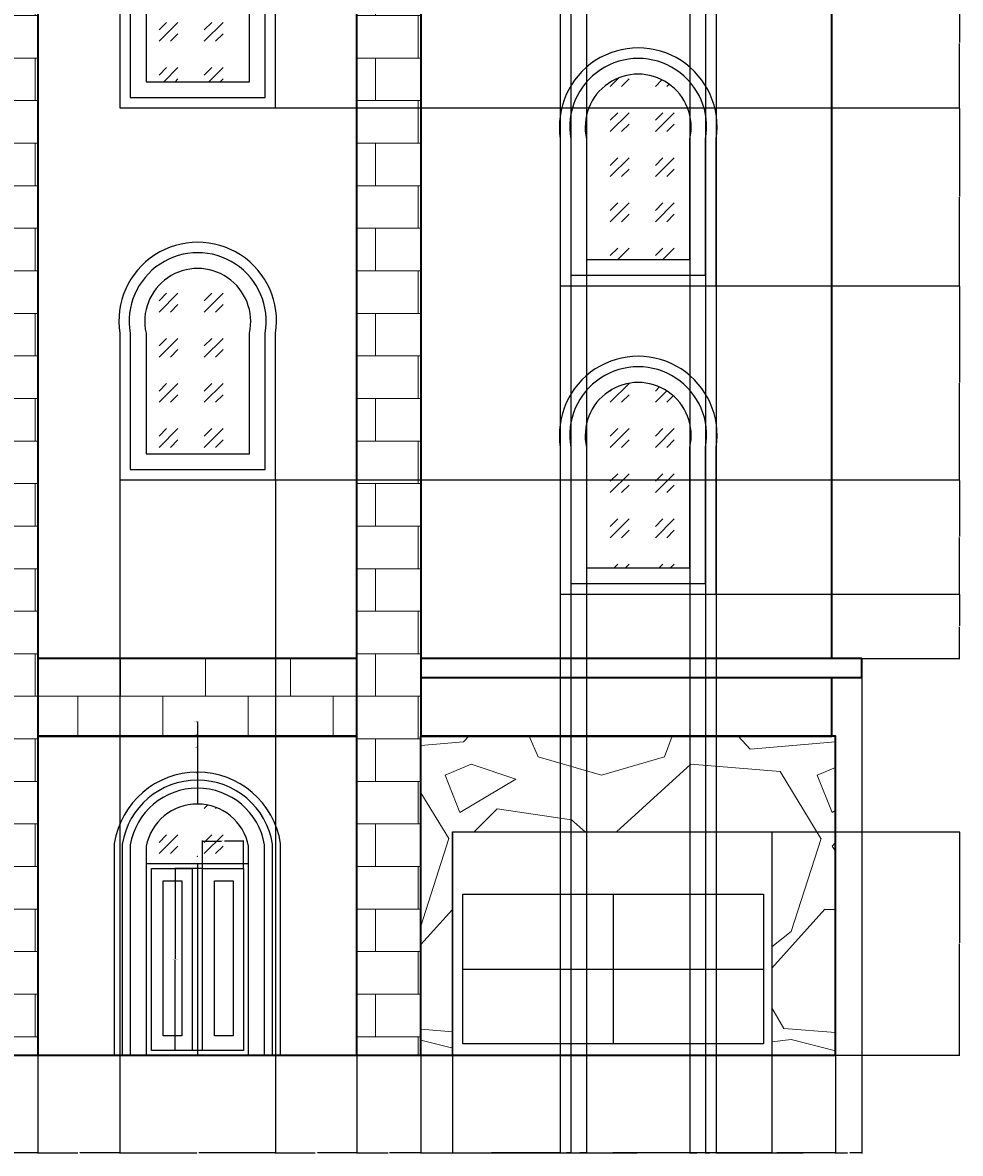
# Model space of a CAD drawing. Units: inches. Extents: x -19 to 556, y -28 to 766.
# Tile 2 of 3: x 203 to 556, y -28 to 397. Entities that reach past the tile are written whole.
import ezdxf

# ---------------------------------------------------------------- set-up
doc = ezdxf.new("R2010")
doc.units = ezdxf.units.IN
doc.header["$MEASUREMENT"] = 0
for name, color, linetype, lineweight in [('A-ANNO-DIMS', 2, 'Continuous', 18), ('A-DOOR', 3, 'Continuous', 25), ('A-ELEV', 7, 'Continuous', 35), ('A-GLAZ', 4, 'Continuous', 25), ('A-GLAZ-PATT', 252, 'Continuous', 13), ('A-WALL-PATT', 8, 'Continuous', 13)]:
    doc.layers.add(name, color=color, linetype=linetype, lineweight=lineweight)
doc.styles.get("Standard").update_dxf_attribs({"font": 'arial.ttf'})
doc.dimstyles.get("Standard").update_dxf_attribs({"dimtxt": 0.18, "dimasz": 0.18, "dimexe": 0.18, "dimexo": 0.0625, "dimgap": 0.09, "dimtad": 0, "dimtih": 1, "dimtoh": 1, "dimdec": 4, "dimzin": 0, "dimdsep": 46, "dimtxsty": 'Standard', "dimcen": 0.09, "dimadec": 0, "dimazin": 0, "dimtfac": 1, "dimtdec": 4, "dimtofl": 0, "dimtmove": 0, "dimatfit": 3, "dimfxl": 1, "dimtolj": 1, "dimtzin": 0, "dimarcsym": 0})
pattern_1 = [(45, (0, 0), (16.97056, 0), [10, -14]), (45, (4.243, 0), (16.97056, 0), [4, -20]), (45, (0, 4.243), (16.97056, 0), [4, -20])]

# ---------------------------------------------------------------- blocks, each defined once
blk = doc.blocks.new('WIN-ARCHED')
for points in [[(65.94, 237.64), (65.94, 182.48), (124.55, 182.48), (124.55, 237.64, 1.168317)], [(69.88, 237.64), (69.88, 186.43), (120.6, 186.43), (120.6, 237.64, 1.194508)], [(75.8, 237.64), (75.8, 192.35), (114.68, 192.35), (114.68, 237.64, 1.253731)]]:
    blk.add_lwpolyline(points, format="xyb", close=True)
blk = doc.blocks.new('DOOR-GARAGE')
for p, q in [((113.34, 69.59), (113.34, 13.35)), ((56.78, 41.47), (169.9, 41.47))]:
    blk.add_line(p, q)
blk.add_lwpolyline([(52.98, 9.07), (52.98, 93.07), (172.98, 93.07), (172.98, 9.07)])
blk.add_lwpolyline([(56.78, 69.59), (169.9, 69.59), (169.9, 13.35), (56.78, 13.35)], close=True)
blk = doc.blocks.new('DOOR-LEAF')
for points in [[(251.66, 79.33), (267.04, 79.33), (267.04, 10.88), (251.66, 10.88)], [(256.13, 74.65), (263.11, 74.65), (263.11, 16.36), (256.13, 16.36)]]:
    blk.add_lwpolyline(points, close=True)
blk = doc.blocks.new('*D6')
at = {"layer": 'A-ANNO-DIMS', "color": 0, "lineweight": -2, "transparency": 16777216}
for p, q in [((270.86, 79.33), (260.47, 79.33)), ((260.65, 79.15), (260.65, 45.29)), ((260.65, 11.06), (260.65, 44.92)), ((270.86, 10.88), (260.47, 10.88))]:
    blk.add_line(p, q, dxfattribs=at)
at = {"layer": 'A-ANNO-DIMS', "color": 0, "transparency": 16777216}
for points in [[(260.62, 79.15), (260.68, 79.15), (260.65, 79.33)], [(260.62, 11.06), (260.68, 11.06), (260.65, 10.88)]]:
    blk.add_solid(points, dxfattribs=at)
at = {"layer": 'Defpoints', "color": 0, "transparency": 16777216}
for p in [(260.65, 79.33), (270.92, 79.33), (270.92, 10.88)]:
    blk.add_point(p, dxfattribs=at)
at = {"layer": 'A-ANNO-DIMS', "color": 0, "transparency": 16777216, "insert": (260.65, 45.1), "char_height": 0.18, "attachment_point": 5}
blk.add_mtext('\\A1;DOOR LEAF 68 TYP.', dxfattribs=at)
blk = doc.blocks.new('*D7')
at = {"layer": 'A-ANNO-DIMS', "color": 0, "lineweight": -2, "transparency": 16777216}
for p, q in [((270.92, 79.39), (270.92, 89.77)), ((271.1, 89.59), (278.09, 89.59)), ((286.12, 89.59), (279.13, 89.59)), ((286.3, 79.39), (286.3, 89.77))]:
    blk.add_line(p, q, dxfattribs=at)
at = {"layer": 'A-ANNO-DIMS', "color": 0, "transparency": 16777216}
for points in [[(271.1, 89.62), (271.1, 89.56), (270.92, 89.59)], [(286.12, 89.62), (286.12, 89.56), (286.3, 89.59)]]:
    blk.add_solid(points, dxfattribs=at)
at = {"layer": 'Defpoints', "color": 0, "transparency": 16777216}
for p in [(286.3, 89.59), (270.92, 79.33), (286.3, 79.33)]:
    blk.add_point(p, dxfattribs=at)
at = {"layer": 'A-ANNO-DIMS', "color": 0, "transparency": 16777216, "insert": (278.61, 89.59), "char_height": 0.18, "attachment_point": 5}
blk.add_mtext('\\A1;15 TYP.', dxfattribs=at)
blk = doc.blocks.new('*D17')
at = {"layer": 'A-ANNO-DIMS', "color": 0, "lineweight": -2, "transparency": 16777216}
for p, q in [((485.05, 93.07), (555.75, 93.07)), ((555.57, 92.89), (555.57, 51.26)), ((555.57, 9.25), (555.57, 50.89)), ((485.05, 9.07), (555.75, 9.07))]:
    blk.add_line(p, q, dxfattribs=at)
at = {"layer": 'A-ANNO-DIMS', "color": 0, "transparency": 16777216}
for points in [[(555.54, 92.89), (555.6, 92.89), (555.57, 93.07)], [(555.54, 9.25), (555.6, 9.25), (555.57, 9.07)]]:
    blk.add_solid(points, dxfattribs=at)
at = {"layer": 'Defpoints', "color": 0, "transparency": 16777216}
for p in [(484.98, 93.07), (555.57, 93.07), (484.98, 9.07)]:
    blk.add_point(p, dxfattribs=at)
at = {"layer": 'A-ANNO-DIMS', "color": 0, "transparency": 16777216, "insert": (555.57, 51.07), "char_height": 0.18, "attachment_point": 5}
blk.add_mtext('\\A1;84', dxfattribs=at)
blk = doc.blocks.new('*D18')
at = {"layer": 'A-ANNO-DIMS', "color": 0, "lineweight": -2, "transparency": 16777216}
for p, q in [((364.98, 93.01), (364.98, -27.86)), ((484.98, 93.01), (484.98, -27.86)), ((365.16, -27.68), (424.7, -27.68)), ((484.8, -27.68), (425.26, -27.68))]:
    blk.add_line(p, q, dxfattribs=at)
at = {"layer": 'A-ANNO-DIMS', "color": 0, "transparency": 16777216}
for points in [[(365.16, -27.65), (365.16, -27.71), (364.98, -27.68)], [(484.8, -27.65), (484.8, -27.71), (484.98, -27.68)]]:
    blk.add_solid(points, dxfattribs=at)
at = {"layer": 'Defpoints', "color": 0, "transparency": 16777216}
for p in [(364.98, 93.07), (484.98, 93.07), (484.98, -27.68)]:
    blk.add_point(p, dxfattribs=at)
at = {"layer": 'A-ANNO-DIMS', "color": 0, "transparency": 16777216, "insert": (424.98, -27.68), "char_height": 0.18, "attachment_point": 5}
blk.add_mtext('\\A1;120', dxfattribs=at)
blk = doc.blocks.new('*D21')
at = {"layer": 'A-ANNO-DIMS', "color": 0, "lineweight": -2, "transparency": 16777216}
for p, q in [((484.98, 9.01), (484.98, -27.86)), ((508.98, 9.01), (508.98, -27.86)), ((485.16, -27.68), (496.76, -27.68)), ((508.8, -27.68), (497.2, -27.68))]:
    blk.add_line(p, q, dxfattribs=at)
at = {"layer": 'A-ANNO-DIMS', "color": 0, "transparency": 16777216}
for points in [[(485.16, -27.65), (485.16, -27.71), (484.98, -27.68)], [(508.8, -27.65), (508.8, -27.71), (508.98, -27.68)]]:
    blk.add_solid(points, dxfattribs=at)
at = {"layer": 'Defpoints', "color": 0, "transparency": 16777216}
for p in [(484.98, 9.07), (508.98, 9.07), (508.98, -27.68)]:
    blk.add_point(p, dxfattribs=at)
at = {"layer": 'A-ANNO-DIMS', "color": 0, "transparency": 16777216, "insert": (496.98, -27.68), "char_height": 0.18, "attachment_point": 5}
blk.add_mtext('\\A1;24', dxfattribs=at)
blk = doc.blocks.new('*D22')
at = {"layer": 'A-ANNO-DIMS', "color": 0, "lineweight": -2, "transparency": 16777216}
for p, q in [((464.13, 182.48), (555.75, 182.48)), ((555.57, 182.3), (555.57, 170.55)), ((555.57, 158.44), (555.57, 170.19)), ((507.68, 158.26), (555.75, 158.26))]:
    blk.add_line(p, q, dxfattribs=at)
at = {"layer": 'A-ANNO-DIMS', "color": 0, "transparency": 16777216}
for points in [[(555.54, 182.3), (555.6, 182.3), (555.57, 182.48)], [(555.54, 158.44), (555.6, 158.44), (555.57, 158.26)]]:
    blk.add_solid(points, dxfattribs=at)
at = {"layer": 'Defpoints', "color": 0, "transparency": 16777216}
for p in [(464.07, 182.48), (555.57, 182.48), (507.61, 158.26)]:
    blk.add_point(p, dxfattribs=at)
at = {"layer": 'A-ANNO-DIMS', "color": 0, "transparency": 16777216, "insert": (555.57, 170.37), "char_height": 0.18, "attachment_point": 5}
blk.add_mtext('\\A1;24.223', dxfattribs=at)
blk = doc.blocks.new('*D23')
at = {"layer": 'A-ANNO-DIMS', "color": 0, "lineweight": -2, "transparency": 16777216}
for p, q in [((298.45, 225.36), (555.75, 225.36)), ((555.57, 225.18), (555.57, 204.1)), ((555.57, 182.66), (555.57, 203.74)), ((464.13, 182.48), (555.75, 182.48))]:
    blk.add_line(p, q, dxfattribs=at)
at = {"layer": 'A-ANNO-DIMS', "color": 0, "transparency": 16777216}
for points in [[(555.54, 225.18), (555.6, 225.18), (555.57, 225.36)], [(555.54, 182.66), (555.6, 182.66), (555.57, 182.48)]]:
    blk.add_solid(points, dxfattribs=at)
at = {"layer": 'Defpoints', "color": 0, "transparency": 16777216}
for p in [(298.39, 225.36), (555.57, 225.36), (464.07, 182.48)]:
    blk.add_point(p, dxfattribs=at)
at = {"layer": 'A-ANNO-DIMS', "color": 0, "transparency": 16777216, "insert": (555.57, 203.92), "char_height": 0.18, "attachment_point": 5}
blk.add_mtext('\\A1;42.88', dxfattribs=at)
blk = doc.blocks.new('*D24')
at = {"layer": 'A-ANNO-DIMS', "color": 0, "lineweight": -2, "transparency": 16777216}
for p, q in [((464.13, 298.43), (555.75, 298.43)), ((555.57, 298.25), (555.57, 262.08)), ((555.57, 225.54), (555.57, 261.71)), ((298.45, 225.36), (555.75, 225.36))]:
    blk.add_line(p, q, dxfattribs=at)
at = {"layer": 'A-ANNO-DIMS', "color": 0, "transparency": 16777216}
for points in [[(555.54, 298.25), (555.6, 298.25), (555.57, 298.43)], [(555.54, 225.54), (555.6, 225.54), (555.57, 225.36)]]:
    blk.add_solid(points, dxfattribs=at)
at = {"layer": 'Defpoints', "color": 0, "transparency": 16777216}
for p in [(464.07, 298.43), (555.57, 298.43), (298.39, 225.36)]:
    blk.add_point(p, dxfattribs=at)
at = {"layer": 'A-ANNO-DIMS', "color": 0, "transparency": 16777216, "insert": (555.57, 261.89), "char_height": 0.18, "attachment_point": 5}
blk.add_mtext('\\A1;73.06', dxfattribs=at)
blk = doc.blocks.new('*D25')
at = {"layer": 'A-ANNO-DIMS', "color": 0, "lineweight": -2, "transparency": 16777216}
for p, q in [((298.45, 365.25), (555.75, 365.25)), ((555.57, 365.07), (555.57, 332.02)), ((555.57, 298.61), (555.57, 331.66)), ((464.13, 298.43), (555.75, 298.43))]:
    blk.add_line(p, q, dxfattribs=at)
at = {"layer": 'A-ANNO-DIMS', "color": 0, "transparency": 16777216}
for points in [[(555.54, 365.07), (555.6, 365.07), (555.57, 365.25)], [(555.54, 298.61), (555.6, 298.61), (555.57, 298.43)]]:
    blk.add_solid(points, dxfattribs=at)
at = {"layer": 'Defpoints', "color": 0, "transparency": 16777216}
for p in [(298.39, 365.25), (555.57, 365.25), (464.07, 298.43)]:
    blk.add_point(p, dxfattribs=at)
at = {"layer": 'A-ANNO-DIMS', "color": 0, "transparency": 16777216, "insert": (555.57, 331.84), "char_height": 0.18, "attachment_point": 5}
blk.add_mtext('\\A1;66.83', dxfattribs=at)
blk = doc.blocks.new('*D26')
at = {"layer": 'A-ANNO-DIMS', "color": 0, "lineweight": -2, "transparency": 16777216}
for p, q in [((464.13, 414.2), (555.75, 414.2)), ((555.57, 414.02), (555.57, 389.91)), ((555.57, 365.43), (555.57, 389.55)), ((298.45, 365.25), (555.75, 365.25))]:
    blk.add_line(p, q, dxfattribs=at)
at = {"layer": 'A-ANNO-DIMS', "color": 0, "transparency": 16777216}
for points in [[(555.54, 414.02), (555.6, 414.02), (555.57, 414.2)], [(555.54, 365.43), (555.6, 365.43), (555.57, 365.25)]]:
    blk.add_solid(points, dxfattribs=at)
at = {"layer": 'Defpoints', "color": 0, "transparency": 16777216}
for p in [(464.07, 414.2), (555.57, 414.2), (298.39, 365.25)]:
    blk.add_point(p, dxfattribs=at)
at = {"layer": 'A-ANNO-DIMS', "color": 0, "transparency": 16777216, "insert": (555.57, 389.73), "char_height": 0.18, "attachment_point": 5}
blk.add_mtext('\\A1;48.95', dxfattribs=at)
blk = doc.blocks.new('*D33')
at = {"layer": 'A-ANNO-DIMS', "color": 0, "lineweight": -2, "transparency": 16777216}
for p, q in [((184.98, 9.01), (184.98, -27.86)), ((208.98, 9.01), (208.98, -27.86)), ((185.16, -27.68), (196.76, -27.68)), ((208.8, -27.68), (197.2, -27.68))]:
    blk.add_line(p, q, dxfattribs=at)
at = {"layer": 'A-ANNO-DIMS', "color": 0, "transparency": 16777216}
for points in [[(185.16, -27.65), (185.16, -27.71), (184.98, -27.68)], [(208.8, -27.65), (208.8, -27.71), (208.98, -27.68)]]:
    blk.add_solid(points, dxfattribs=at)
at = {"layer": 'Defpoints', "color": 0, "transparency": 16777216}
for p in [(184.98, 9.07), (208.98, 9.07), (208.98, -27.68)]:
    blk.add_point(p, dxfattribs=at)
at = {"layer": 'A-ANNO-DIMS', "color": 0, "transparency": 16777216, "insert": (196.98, -27.68), "char_height": 0.18, "attachment_point": 5}
blk.add_mtext('\\A1;24', dxfattribs=at)
blk = doc.blocks.new('*D34')
at = {"layer": 'A-ANNO-DIMS', "color": 0, "lineweight": -2, "transparency": 16777216}
for p, q in [((239.78, 225.3), (239.78, -27.86)), ((208.98, 9.01), (208.98, -27.86)), ((209.16, -27.68), (223.99, -27.68)), ((239.6, -27.68), (224.77, -27.68))]:
    blk.add_line(p, q, dxfattribs=at)
at = {"layer": 'A-ANNO-DIMS', "color": 0, "transparency": 16777216}
for points in [[(209.16, -27.65), (209.16, -27.71), (208.98, -27.68)], [(239.6, -27.65), (239.6, -27.71), (239.78, -27.68)]]:
    blk.add_solid(points, dxfattribs=at)
at = {"layer": 'Defpoints', "color": 0, "transparency": 16777216}
for p in [(239.78, 225.36), (208.98, 9.07), (239.78, -27.68)]:
    blk.add_point(p, dxfattribs=at)
at = {"layer": 'A-ANNO-DIMS', "color": 0, "transparency": 16777216, "insert": (224.38, -27.68), "char_height": 0.18, "attachment_point": 5}
blk.add_mtext('\\A1;30.79', dxfattribs=at)
blk = doc.blocks.new('*D35')
at = {"layer": 'A-ANNO-DIMS', "color": 0, "lineweight": -2, "transparency": 16777216}
for p, q in [((239.78, 225.3), (239.78, -27.86)), ((298.39, 225.3), (298.39, -27.86)), ((239.96, -27.68), (268.71, -27.68)), ((298.21, -27.68), (269.46, -27.68))]:
    blk.add_line(p, q, dxfattribs=at)
at = {"layer": 'A-ANNO-DIMS', "color": 0, "transparency": 16777216}
for points in [[(239.96, -27.65), (239.96, -27.71), (239.78, -27.68)], [(298.21, -27.65), (298.21, -27.71), (298.39, -27.68)]]:
    blk.add_solid(points, dxfattribs=at)
at = {"layer": 'Defpoints', "color": 0, "transparency": 16777216}
for p in [(239.78, 225.36), (298.39, 225.36), (298.39, -27.68)]:
    blk.add_point(p, dxfattribs=at)
at = {"layer": 'A-ANNO-DIMS', "color": 0, "transparency": 16777216, "insert": (269.08, -27.68), "char_height": 0.18, "attachment_point": 5}
blk.add_mtext('\\A1;58.61', dxfattribs=at)
blk = doc.blocks.new('*D36')
at = {"layer": 'A-ANNO-DIMS', "color": 0, "lineweight": -2, "transparency": 16777216}
for p, q in [((298.39, 225.3), (298.39, -27.86)), ((328.98, 9.01), (328.98, -27.86)), ((298.57, -27.68), (313.22, -27.68)), ((328.8, -27.68), (314.15, -27.68))]:
    blk.add_line(p, q, dxfattribs=at)
at = {"layer": 'A-ANNO-DIMS', "color": 0, "transparency": 16777216}
for points in [[(298.57, -27.65), (298.57, -27.71), (298.39, -27.68)], [(328.8, -27.65), (328.8, -27.71), (328.98, -27.68)]]:
    blk.add_solid(points, dxfattribs=at)
at = {"layer": 'Defpoints', "color": 0, "transparency": 16777216}
for p in [(298.39, 225.36), (328.98, 9.07), (328.98, -27.68)]:
    blk.add_point(p, dxfattribs=at)
at = {"layer": 'A-ANNO-DIMS', "color": 0, "transparency": 16777216, "insert": (313.69, -27.68), "char_height": 0.18, "attachment_point": 5}
blk.add_mtext('\\A1;30.593', dxfattribs=at)
blk = doc.blocks.new('*D37')
at = {"layer": 'A-ANNO-DIMS', "color": 0, "lineweight": -2, "transparency": 16777216}
for p, q in [((328.98, 9.01), (328.98, -27.86)), ((352.98, 9.01), (352.98, -27.86)), ((329.16, -27.68), (340.76, -27.68)), ((352.8, -27.68), (341.2, -27.68))]:
    blk.add_line(p, q, dxfattribs=at)
at = {"layer": 'A-ANNO-DIMS', "color": 0, "transparency": 16777216}
for points in [[(329.16, -27.65), (329.16, -27.71), (328.98, -27.68)], [(352.8, -27.65), (352.8, -27.71), (352.98, -27.68)]]:
    blk.add_solid(points, dxfattribs=at)
at = {"layer": 'Defpoints', "color": 0, "transparency": 16777216}
for p in [(328.98, 9.07), (352.98, 9.07), (352.98, -27.68)]:
    blk.add_point(p, dxfattribs=at)
at = {"layer": 'A-ANNO-DIMS', "color": 0, "transparency": 16777216, "insert": (340.98, -27.68), "char_height": 0.18, "attachment_point": 5}
blk.add_mtext('\\A1;24', dxfattribs=at)
blk = doc.blocks.new('*D38')
at = {"layer": 'A-ANNO-DIMS', "color": 0, "lineweight": -2, "transparency": 16777216}
for p, q in [((405.46, 182.42), (405.46, -27.86)), ((352.98, 9.01), (352.98, -27.86)), ((353.16, -27.68), (378.83, -27.68)), ((405.28, -27.68), (379.61, -27.68))]:
    blk.add_line(p, q, dxfattribs=at)
at = {"layer": 'A-ANNO-DIMS', "color": 0, "transparency": 16777216}
for points in [[(353.16, -27.65), (353.16, -27.71), (352.98, -27.68)], [(405.28, -27.65), (405.28, -27.71), (405.46, -27.68)]]:
    blk.add_solid(points, dxfattribs=at)
at = {"layer": 'Defpoints', "color": 0, "transparency": 16777216}
for p in [(405.46, 182.48), (352.98, 9.07), (405.46, -27.68)]:
    blk.add_point(p, dxfattribs=at)
at = {"layer": 'A-ANNO-DIMS', "color": 0, "transparency": 16777216, "insert": (379.22, -27.68), "char_height": 0.18, "attachment_point": 5}
blk.add_mtext('\\A1;52.47', dxfattribs=at)
blk = doc.blocks.new('*D39')
at = {"layer": 'A-ANNO-DIMS', "color": 0, "lineweight": -2, "transparency": 16777216}
for p, q in [((405.46, 182.42), (405.46, -27.86)), ((464.07, 182.42), (464.07, -27.86)), ((405.64, -27.68), (434.39, -27.68)), ((463.89, -27.68), (435.14, -27.68))]:
    blk.add_line(p, q, dxfattribs=at)
at = {"layer": 'A-ANNO-DIMS', "color": 0, "transparency": 16777216}
for points in [[(405.64, -27.65), (405.64, -27.71), (405.46, -27.68)], [(463.89, -27.65), (463.89, -27.71), (464.07, -27.68)]]:
    blk.add_solid(points, dxfattribs=at)
at = {"layer": 'Defpoints', "color": 0, "transparency": 16777216}
for p in [(405.46, 182.48), (464.07, 182.48), (464.07, -27.68)]:
    blk.add_point(p, dxfattribs=at)
at = {"layer": 'A-ANNO-DIMS', "color": 0, "transparency": 16777216, "insert": (434.76, -27.68), "char_height": 0.18, "attachment_point": 5}
blk.add_mtext('\\A1;58.61', dxfattribs=at)
blk = doc.blocks.new('*D40')
at = {"layer": 'A-ANNO-DIMS', "color": 0, "lineweight": -2, "transparency": 16777216}
for p, q in [((464.07, 182.42), (464.07, -27.86)), ((508.98, 9.01), (508.98, -27.86)), ((464.25, -27.68), (486.15, -27.68)), ((508.8, -27.68), (486.91, -27.68))]:
    blk.add_line(p, q, dxfattribs=at)
at = {"layer": 'A-ANNO-DIMS', "color": 0, "transparency": 16777216}
for points in [[(464.25, -27.65), (464.25, -27.71), (464.07, -27.68)], [(508.8, -27.65), (508.8, -27.71), (508.98, -27.68)]]:
    blk.add_solid(points, dxfattribs=at)
at = {"layer": 'Defpoints', "color": 0, "transparency": 16777216}
for p in [(464.07, 182.48), (508.98, 9.07), (508.98, -27.68)]:
    blk.add_point(p, dxfattribs=at)
at = {"layer": 'A-ANNO-DIMS', "color": 0, "transparency": 16777216, "insert": (486.53, -27.68), "char_height": 0.18, "attachment_point": 5}
blk.add_mtext('\\A1;44.91', dxfattribs=at)
blk = doc.blocks.new('*D41')
at = {"layer": 'A-ANNO-DIMS', "color": 0, "lineweight": -2, "transparency": 16777216}
for p, q in [((518.82, 150.98), (518.82, -27.86)), ((508.98, 9.01), (508.98, -27.86)), ((509.16, -27.68), (513.51, -27.68)), ((518.64, -27.68), (514.3, -27.68))]:
    blk.add_line(p, q, dxfattribs=at)
at = {"layer": 'A-ANNO-DIMS', "color": 0, "transparency": 16777216}
for points in [[(509.16, -27.65), (509.16, -27.71), (508.98, -27.68)], [(518.64, -27.65), (518.64, -27.71), (518.82, -27.68)]]:
    blk.add_solid(points, dxfattribs=at)
at = {"layer": 'Defpoints', "color": 0, "transparency": 16777216}
for p in [(518.82, 151.04), (508.98, 9.07), (518.82, -27.68)]:
    blk.add_point(p, dxfattribs=at)
at = {"layer": 'A-ANNO-DIMS', "color": 0, "transparency": 16777216, "insert": (513.9, -27.68), "char_height": 0.18, "attachment_point": 5}
blk.add_mtext('\\A1;9.836', dxfattribs=at)
blk = doc.blocks.new('*D42')
at = {"layer": 'A-ANNO-DIMS', "color": 0, "lineweight": -2, "transparency": 16777216}
for p, q in [((409.4, 540.54), (409.4, -27.86)), ((405.46, 536.6), (405.46, -27.86)), ((405.64, -27.68), (407.04, -27.68)), ((409.22, -27.68), (407.82, -27.68))]:
    blk.add_line(p, q, dxfattribs=at)
at = {"layer": 'A-ANNO-DIMS', "color": 0, "transparency": 16777216}
for points in [[(405.64, -27.65), (405.64, -27.71), (405.46, -27.68)], [(409.22, -27.65), (409.22, -27.71), (409.4, -27.68)]]:
    blk.add_solid(points, dxfattribs=at)
at = {"layer": 'Defpoints', "color": 0, "transparency": 16777216}
for p in [(409.4, 540.61), (405.46, 536.66), (409.4, -27.68)]:
    blk.add_point(p, dxfattribs=at)
at = {"layer": 'A-ANNO-DIMS', "color": 0, "transparency": 16777216, "insert": (407.43, -27.68), "char_height": 0.18, "attachment_point": 5}
blk.add_mtext('\\A1;3.946', dxfattribs=at)
blk = doc.blocks.new('*D43')
at = {"layer": 'A-ANNO-DIMS', "color": 0, "lineweight": -2, "transparency": 16777216}
for p, q in [((415.32, 546.46), (415.32, -27.86)), ((409.4, 540.54), (409.4, -27.86)), ((409.58, -27.68), (411.97, -27.68)), ((415.14, -27.68), (412.76, -27.68))]:
    blk.add_line(p, q, dxfattribs=at)
at = {"layer": 'A-ANNO-DIMS', "color": 0, "transparency": 16777216}
for points in [[(409.58, -27.65), (409.58, -27.71), (409.4, -27.68)], [(415.14, -27.65), (415.14, -27.71), (415.32, -27.68)]]:
    blk.add_solid(points, dxfattribs=at)
at = {"layer": 'Defpoints', "color": 0, "transparency": 16777216}
for p in [(415.32, 546.52), (409.4, 540.61), (415.32, -27.68)]:
    blk.add_point(p, dxfattribs=at)
at = {"layer": 'A-ANNO-DIMS', "color": 0, "transparency": 16777216, "insert": (412.36, -27.68), "char_height": 0.18, "attachment_point": 5}
blk.add_mtext('\\A1;5.919', dxfattribs=at)
blk = doc.blocks.new('*D44')
at = {"layer": 'A-ANNO-DIMS', "color": 0, "lineweight": -2, "transparency": 16777216}
for p, q in [((415.32, 546.46), (415.32, -27.86)), ((454.21, 546.46), (454.21, -27.86)), ((415.5, -27.68), (434.37, -27.68)), ((454.03, -27.68), (435.16, -27.68))]:
    blk.add_line(p, q, dxfattribs=at)
at = {"layer": 'A-ANNO-DIMS', "color": 0, "transparency": 16777216}
for points in [[(415.5, -27.65), (415.5, -27.71), (415.32, -27.68)], [(454.03, -27.65), (454.03, -27.71), (454.21, -27.68)]]:
    blk.add_solid(points, dxfattribs=at)
at = {"layer": 'Defpoints', "color": 0, "transparency": 16777216}
for p in [(415.32, 546.52), (454.21, 546.52), (454.21, -27.68)]:
    blk.add_point(p, dxfattribs=at)
at = {"layer": 'A-ANNO-DIMS', "color": 0, "transparency": 16777216, "insert": (434.76, -27.68), "char_height": 0.18, "attachment_point": 5}
blk.add_mtext('\\A1;38.88', dxfattribs=at)
blk = doc.blocks.new('*D45')
at = {"layer": 'A-ANNO-DIMS', "color": 0, "lineweight": -2, "transparency": 16777216}
for p, q in [((454.21, 546.46), (454.21, -27.86)), ((460.12, 540.54), (460.12, -27.86)), ((454.39, -27.68), (456.77, -27.68)), ((459.94, -27.68), (457.56, -27.68))]:
    blk.add_line(p, q, dxfattribs=at)
at = {"layer": 'A-ANNO-DIMS', "color": 0, "transparency": 16777216}
for points in [[(454.39, -27.65), (454.39, -27.71), (454.21, -27.68)], [(459.94, -27.65), (459.94, -27.71), (460.12, -27.68)]]:
    blk.add_solid(points, dxfattribs=at)
at = {"layer": 'Defpoints', "color": 0, "transparency": 16777216}
for p in [(454.21, 546.52), (460.12, 540.61), (460.12, -27.68)]:
    blk.add_point(p, dxfattribs=at)
at = {"layer": 'A-ANNO-DIMS', "color": 0, "transparency": 16777216, "insert": (457.16, -27.68), "char_height": 0.18, "attachment_point": 5}
blk.add_mtext('\\A1;5.919', dxfattribs=at)
blk = doc.blocks.new('*D46')
at = {"layer": 'A-ANNO-DIMS', "color": 0, "lineweight": -2, "transparency": 16777216}
for p, q in [((460.12, 540.54), (460.12, -27.86)), ((464.07, 536.6), (464.07, -27.86)), ((460.3, -27.68), (461.7, -27.68)), ((463.89, -27.68), (462.49, -27.68))]:
    blk.add_line(p, q, dxfattribs=at)
at = {"layer": 'A-ANNO-DIMS', "color": 0, "transparency": 16777216}
for points in [[(460.3, -27.65), (460.3, -27.71), (460.12, -27.68)], [(463.89, -27.65), (463.89, -27.71), (464.07, -27.68)]]:
    blk.add_solid(points, dxfattribs=at)
at = {"layer": 'Defpoints', "color": 0, "transparency": 16777216}
for p in [(460.12, 540.61), (464.07, 536.66), (464.07, -27.68)]:
    blk.add_point(p, dxfattribs=at)
at = {"layer": 'A-ANNO-DIMS', "color": 0, "transparency": 16777216, "insert": (462.1, -27.68), "char_height": 0.18, "attachment_point": 5}
blk.add_mtext('\\A1;3.946', dxfattribs=at)
blk = doc.blocks.new('*D54')
at = {"layer": 'A-ANNO-DIMS', "color": 0, "lineweight": -2, "transparency": 16777216}
for p, q in [((268.8, 134.46), (268.98, 134.46)), ((268.98, 134.46), (268.98, 115.67)), ((268.89, 83.86), (269.07, 83.86)), ((268.98, 83.77), (268.98, 83.95))]:
    blk.add_line(p, q, dxfattribs=at)
at = {"layer": 'A-ANNO-DIMS', "color": 0, "transparency": 16777216}
blk.add_solid([(269.01, 115.67), (268.95, 115.67), (268.98, 115.49)], dxfattribs=at)
at = {"layer": 'Defpoints', "color": 0, "transparency": 16777216}
for p in [(268.98, 115.49), (268.98, 83.86)]:
    blk.add_point(p, dxfattribs=at)
at = {"layer": 'A-ANNO-DIMS', "color": 0, "transparency": 16777216, "insert": (268.25, 134.46), "char_height": 0.18, "attachment_point": 5}
blk.add_mtext('\\A1;R31.625', dxfattribs=at)
blk = doc.blocks.new('*D55')
at = {"layer": 'A-ANNO-DIMS', "color": 0, "lineweight": -2, "transparency": 16777216}
for p, q in [((268.8, 129.66), (268.98, 129.66)), ((268.98, 129.66), (268.98, 112.67)), ((268.89, 83.86), (269.07, 83.86)), ((268.98, 83.77), (268.98, 83.95))]:
    blk.add_line(p, q, dxfattribs=at)
at = {"layer": 'A-ANNO-DIMS', "color": 0, "transparency": 16777216}
blk.add_solid([(269.01, 112.67), (268.95, 112.67), (268.98, 112.49)], dxfattribs=at)
at = {"layer": 'Defpoints', "color": 0, "transparency": 16777216}
for p in [(268.98, 112.49), (268.98, 83.86)]:
    blk.add_point(p, dxfattribs=at)
at = {"layer": 'A-ANNO-DIMS', "color": 0, "transparency": 16777216, "insert": (268.25, 129.66), "char_height": 0.18, "attachment_point": 5}
blk.add_mtext('\\A1;R28.625', dxfattribs=at)
blk = doc.blocks.new('*D56')
at = {"layer": 'A-ANNO-DIMS', "color": 0, "lineweight": -2, "transparency": 16777216}
for p, q in [((268.8, 124.86), (268.98, 124.86)), ((268.98, 124.86), (268.98, 109.67)), ((268.89, 83.86), (269.07, 83.86)), ((268.98, 83.77), (268.98, 83.95))]:
    blk.add_line(p, q, dxfattribs=at)
at = {"layer": 'A-ANNO-DIMS', "color": 0, "transparency": 16777216}
blk.add_solid([(269.01, 109.67), (268.95, 109.67), (268.98, 109.49)], dxfattribs=at)
at = {"layer": 'Defpoints', "color": 0, "transparency": 16777216}
for p in [(268.98, 109.49), (268.98, 83.86)]:
    blk.add_point(p, dxfattribs=at)
at = {"layer": 'A-ANNO-DIMS', "color": 0, "transparency": 16777216, "insert": (268.25, 124.86), "char_height": 0.18, "attachment_point": 5}
blk.add_mtext('\\A1;R25.625', dxfattribs=at)
blk = doc.blocks.new('*D57')
at = {"layer": 'A-ANNO-DIMS', "color": 0, "lineweight": -2, "transparency": 16777216}
for p, q in [((268.8, 115.26), (268.98, 115.26)), ((268.98, 115.26), (268.98, 103.67)), ((268.89, 83.86), (269.07, 83.86)), ((268.98, 83.77), (268.98, 83.95))]:
    blk.add_line(p, q, dxfattribs=at)
at = {"layer": 'A-ANNO-DIMS', "color": 0, "transparency": 16777216}
blk.add_solid([(269.01, 103.67), (268.95, 103.67), (268.98, 103.49)], dxfattribs=at)
at = {"layer": 'Defpoints', "color": 0, "transparency": 16777216}
for p in [(268.98, 103.49), (268.98, 83.86)]:
    blk.add_point(p, dxfattribs=at)
at = {"layer": 'A-ANNO-DIMS', "color": 0, "transparency": 16777216, "insert": (268.25, 115.26), "char_height": 0.18, "attachment_point": 5}
blk.add_mtext('\\A1;R19.625', dxfattribs=at)
blk = doc.blocks.new('*D58')
at = {"layer": 'A-ANNO-DIMS', "color": 0, "lineweight": -2, "transparency": 16777216}
for p, q in [((268.8, 134.46), (268.98, 134.46)), ((268.98, 134.46), (268.98, 115.67)), ((268.89, 83.86), (269.07, 83.86)), ((268.98, 83.77), (268.98, 83.95))]:
    blk.add_line(p, q, dxfattribs=at)
at = {"layer": 'A-ANNO-DIMS', "color": 0, "transparency": 16777216}
blk.add_solid([(269.01, 115.67), (268.95, 115.67), (268.98, 115.49)], dxfattribs=at)
at = {"layer": 'Defpoints', "color": 0, "transparency": 16777216}
for p in [(268.98, 115.49), (268.98, 83.86)]:
    blk.add_point(p, dxfattribs=at)
at = {"layer": 'A-ANNO-DIMS', "color": 0, "transparency": 16777216, "insert": (268.25, 134.46), "char_height": 0.18, "attachment_point": 5}
blk.add_mtext('\\A1;R31.625', dxfattribs=at)
blk = doc.blocks.new('*D59')
at = {"layer": 'A-ANNO-DIMS', "color": 0, "lineweight": -2, "transparency": 16777216}
for p, q in [((268.8, 129.66), (268.98, 129.66)), ((268.98, 129.66), (268.98, 112.67)), ((268.89, 83.86), (269.07, 83.86)), ((268.98, 83.77), (268.98, 83.95))]:
    blk.add_line(p, q, dxfattribs=at)
at = {"layer": 'A-ANNO-DIMS', "color": 0, "transparency": 16777216}
blk.add_solid([(269.01, 112.67), (268.95, 112.67), (268.98, 112.49)], dxfattribs=at)
at = {"layer": 'Defpoints', "color": 0, "transparency": 16777216}
for p in [(268.98, 112.49), (268.98, 83.86)]:
    blk.add_point(p, dxfattribs=at)
at = {"layer": 'A-ANNO-DIMS', "color": 0, "transparency": 16777216, "insert": (268.25, 129.66), "char_height": 0.18, "attachment_point": 5}
blk.add_mtext('\\A1;R28.625', dxfattribs=at)
blk = doc.blocks.new('*D60')
at = {"layer": 'A-ANNO-DIMS', "color": 0, "lineweight": -2, "transparency": 16777216}
for p, q in [((268.8, 124.86), (268.98, 124.86)), ((268.98, 124.86), (268.98, 109.67)), ((268.89, 83.86), (269.07, 83.86)), ((268.98, 83.77), (268.98, 83.95))]:
    blk.add_line(p, q, dxfattribs=at)
at = {"layer": 'A-ANNO-DIMS', "color": 0, "transparency": 16777216}
blk.add_solid([(269.01, 109.67), (268.95, 109.67), (268.98, 109.49)], dxfattribs=at)
at = {"layer": 'Defpoints', "color": 0, "transparency": 16777216}
for p in [(268.98, 109.49), (268.98, 83.86)]:
    blk.add_point(p, dxfattribs=at)
at = {"layer": 'A-ANNO-DIMS', "color": 0, "transparency": 16777216, "insert": (268.25, 124.86), "char_height": 0.18, "attachment_point": 5}
blk.add_mtext('\\A1;R25.625', dxfattribs=at)
blk = doc.blocks.new('*D61')
at = {"layer": 'A-ANNO-DIMS', "color": 0, "lineweight": -2, "transparency": 16777216}
for p, q in [((268.8, 115.26), (268.98, 115.26)), ((268.98, 115.26), (268.98, 103.67)), ((268.89, 83.86), (269.07, 83.86)), ((268.98, 83.77), (268.98, 83.95))]:
    blk.add_line(p, q, dxfattribs=at)
at = {"layer": 'A-ANNO-DIMS', "color": 0, "transparency": 16777216}
blk.add_solid([(269.01, 103.67), (268.95, 103.67), (268.98, 103.49)], dxfattribs=at)
at = {"layer": 'Defpoints', "color": 0, "transparency": 16777216}
for p in [(268.98, 103.49), (268.98, 83.86)]:
    blk.add_point(p, dxfattribs=at)
at = {"layer": 'A-ANNO-DIMS', "color": 0, "transparency": 16777216, "insert": (268.25, 115.26), "char_height": 0.18, "attachment_point": 5}
blk.add_mtext('\\A1;R19.625', dxfattribs=at)

msp = doc.modelspace()

# ---------------------------------------------------------------- hatches: boundary and pattern name
at = {"layer": 'A-GLAZ-PATT'}
h = msp.add_hatch(dxfattribs=at)
h.set_pattern_fill('GOST_GLASS', color=256, scale=2)
h.set_pattern_definition(pattern_1)
h.paths.add_polyline_path([(114.6834, 591.8123, 1.25373075), (75.801, 591.8123), (75.801, 546.5249), (114.6834, 546.5249)])
h.paths.add_polyline_path([(454.2051, 591.8123, 1.25373075), (415.3227, 591.8123), (415.3227, 546.5249), (454.2051, 546.5249)])
h.paths.add_polyline_path([(288.5244, 564.1792, 1.25373075), (249.6421, 564.1792), (249.6421, 518.8919), (288.5244, 518.8919)])
h.paths.add_polyline_path([(114.6834, 469.356, 1.25373075), (75.801, 469.356), (75.801, 424.0687), (114.6834, 424.0687)])
h.paths.add_polyline_path([(288.5244, 420.4043, 1.25373075), (249.6421, 420.4043), (249.6421, 375.1169), (288.5244, 375.1169)])
h.paths.add_polyline_path([(454.2051, 469.356, 1.25373075), (415.3227, 469.356), (415.3227, 424.0687), (454.2051, 424.0687)])
h.paths.add_polyline_path([(454.2051, 353.5792, 1.25373075), (415.3227, 353.5792), (415.3227, 308.2919), (454.2051, 308.2919)])
h.paths.add_polyline_path([(454.2051, 237.6357, 1.25373075), (415.3227, 237.6357), (415.3227, 192.3483), (454.2051, 192.3483)])
h.paths.add_polyline_path([(288.5244, 280.5161, 1.25373075), (249.6421, 280.5161), (249.6421, 235.2288), (288.5244, 235.2288)])
h.paths.add_polyline_path([(114.6834, 237.6357, 1.25373075), (75.801, 237.6357), (75.801, 192.3483), (114.6834, 192.3483)])
h.paths.add_polyline_path([(114.6834, 353.5792, 1.25373075), (75.801, 353.5792), (75.801, 308.2919), (114.6834, 308.2919)])
h = msp.add_hatch(dxfattribs=at)
h.set_pattern_fill('GOST_GLASS', color=256, scale=2)
h.set_pattern_definition(pattern_1)
h.paths.add_polyline_path([(249.7265, 87.6475), (249.7265, 81.2077), (288.2402, 81.2077), (288.2402, 87.6475, 0.82262604)])
at = {"layer": 'A-WALL-PATT'}
h = msp.add_hatch(dxfattribs=at)
h.set_pattern_fill('AR-B816', color=256, scale=2)
h.paths.add_polyline_path([(208.9833, 669.0741), (184.9833, 669.0741), (184.9833, 129.0741), (184.9833, 9.0741), (208.9833, 9.0741), (208.9833, 129.0741)])
h.paths.add_polyline_path([(352.9833, 669.0741), (328.9833, 669.0741), (328.9833, 129.0741), (328.9833, 9.0741), (352.9833, 9.0741), (352.9833, 129.0741)])
h = msp.add_hatch(dxfattribs=at)
h.set_pattern_fill('AR-B816', color=256, scale=2)
h.paths.add_polyline_path([(328.9833, 158.26), (208.9833, 158.26), (208.9833, 129.0741), (328.9833, 129.0741)])
h = msp.add_hatch(dxfattribs=at)
h.set_pattern_fill('GRAVEL', color=256, scale=140)
h.paths.add_polyline_path([(184.9833, 129.0741), (28.9833, 129.0741), (28.9833, 9.0741), (52.9833, 9.0741), (52.9833, 93.0741), (172.9833, 93.0741), (172.9833, 9.0741), (184.9833, 9.0741)])
h.paths.add_polyline_path([(508.9833, 129.0741), (352.9833, 129.0741), (352.9833, 9.0741), (364.9833, 9.0741), (364.9833, 93.0741), (484.9833, 93.0741), (484.9833, 9.0741), (508.9833, 9.0741)])

# ---------------------------------------------------------------- linework, layer by layer
at = {"layer": 'A-DOOR'}
for p, q in [((249.7265, 81.2077), (288.2402, 81.2077)), ((268.9833, 81.2077), (268.9833, 9.0741))]:
    msp.add_line(p, q, dxfattribs=at)
for points in [[(300.2402, 9.0741), (300.2402, 88.6756, 0.8578296), (237.7265, 88.6756), (237.7265, 9.0741)], [(297.2402, 9.0741), (297.2402, 88.4403, 0.85106374), (240.7265, 88.4403), (240.7265, 9.0741)], [(294.2402, 9.0741), (294.2402, 88.1922, 0.84319639), (243.7265, 88.1922), (243.7265, 9.0741)], [(288.2402, 9.0741), (288.2402, 87.6475, 0.82262604), (249.7265, 87.6475), (249.7265, 9.0741)]]:
    msp.add_lwpolyline(points, format="xyb", dxfattribs=at)
at = {"layer": 'A-ELEV'}
for p, q in [((328.9833, 129.0741), (328.9833, 669.0741)), ((352.9833, 669.0741), (352.9833, 129.0741)), ((518.8195, 158.26), (507.6136, 158.26)), ((518.8195, 151.0378), (518.8195, 158.26)), ((352.9833, 151.0378), (518.8195, 151.0378)), ((328.9833, 129.0741), (208.9833, 129.0741)), ((328.9833, 9.0741), (328.9833, 129.0741))]:
    msp.add_line(p, q, dxfattribs=at)
for points in [[(507.6136, 158.26), (507.6136, 669.0741), (28.9833, 669.0741), (28.9833, 158.26)], [(208.9833, 669.0741), (208.9833, 129.0741), (208.9833, 9.0741)], [(328.9833, 158.26), (208.9833, 158.26)], [(507.6136, 158.26), (352.9833, 158.26)], [(352.9833, 129.0741), (507.6136, 129.0741), (507.6136, 151.0378)], [(352.9833, 9.0741), (352.9833, 129.0741), (507.6136, 129.0741), (507.6136, 151.0378)], [(184.9833, 129.0741), (28.9833, 129.0741), (28.9833, 9.0741), (508.9833, 9.0741), (508.9833, 129.0741), (352.9833, 129.0741)]]:
    msp.add_lwpolyline(points, dxfattribs=at)
msp.add_lwpolyline([(328.9833, 129.0741), (208.9833, 129.0741)], close=True, dxfattribs=at)

# ---------------------------------------------------------------- block references
at = {"layer": 'A-DOOR'}
for name, p in [('DOOR-GARAGE', (312, 0)), ('DOOR-LEAF', (0, 0)), ('DOOR-LEAF', (19.2569, 0))]:
    msp.add_blockref(name, p, dxfattribs=at)
at = {"layer": 'A-GLAZ'}
for p in [(173.841, 182.7686), (339.5217, 115.9436), (173.841, 42.8805), (339.5217, 0)]:
    msp.add_blockref('WIN-ARCHED', p, dxfattribs=at)

# ---------------------------------------------------------------- dimensions: what is measured, and where the dimension line sits
at = {"layer": 'A-ANNO-DIMS'}
for base, p1, p2, override, picture, middle in [((415.3227, -27.6759), (409.4034, 540.6055), (415.3227, 546.5249), {"dimdec": 3, "dimlfac": 1, "dimrnd": 0, "dimzin": 0, "dimdsep": 46, "dimlunit": 2}, '*D43', (412.3631, -27.6759)), ((454.2051, -27.6759), (415.3227, 546.5249), (454.2051, 546.5249), {"dimdec": 2, "dimlfac": 1, "dimrnd": 0, "dimzin": 0, "dimdsep": 46, "dimlunit": 2}, '*D44', (434.7639, -27.6759)), ((460.1245, -27.6759), (454.2051, 546.5249), (460.1245, 540.6055), {"dimdec": 3, "dimlfac": 1, "dimrnd": 0, "dimzin": 0, "dimdsep": 46, "dimlunit": 2}, '*D45', (457.1648, -27.6759)), ((409.4034, -27.6759), (405.4571, 536.6593), (409.4034, 540.6055), {"dimdec": 3, "dimlfac": 1, "dimrnd": 0, "dimzin": 0, "dimdsep": 46, "dimlunit": 2}, '*D42', (407.4302, -27.6759)), ((464.0708, -27.6759), (460.1245, 540.6055), (464.0708, 536.6593), {"dimdec": 3, "dimlfac": 1, "dimrnd": 0, "dimzin": 0, "dimdsep": 46, "dimlunit": 2}, '*D46', (462.0976, -27.6759)), ((239.7764, -27.6759), (208.9833, 9.0741), (239.7764, 225.3631), {"dimdec": 2, "dimlfac": 1, "dimrnd": 0, "dimzin": 0, "dimdsep": 46, "dimlunit": 2}, '*D34', (224.3799, -27.6759)), ((298.3901, -27.6759), (239.7764, 225.3631), (298.3901, 225.3631), {"dimdec": 2, "dimlfac": 1, "dimrnd": 0, "dimzin": 0, "dimdsep": 46, "dimlunit": 2}, '*D35', (269.0832, -27.6759)), ((328.9833, -27.6759), (298.3901, 225.3631), (328.9833, 9.0741), {"dimdec": 3, "dimlfac": 1, "dimrnd": 0, "dimzin": 0, "dimdsep": 46, "dimlunit": 2}, '*D36', (313.6867, -27.6759)), ((405.4571, -27.6759), (352.9833, 9.0741), (405.4571, 182.4827), {"dimdec": 2, "dimlfac": 1, "dimrnd": 0, "dimzin": 0, "dimdsep": 46, "dimlunit": 2}, '*D38', (379.2202, -27.6759)), ((464.0708, -27.6759), (405.4571, 182.4827), (464.0708, 182.4827), {"dimdec": 2, "dimlfac": 1, "dimrnd": 0, "dimzin": 0, "dimdsep": 46, "dimlunit": 2}, '*D39', (434.7639, -27.6759)), ((508.9833, -27.6759), (464.0708, 182.4827), (508.9833, 9.0741), {"dimdec": 2, "dimlfac": 1, "dimrnd": 0, "dimzin": 0, "dimdsep": 46, "dimlunit": 2}, '*D40', (486.527, -27.6759)), ((518.8195, -27.6759), (508.9833, 9.0741), (518.8195, 151.0378), {"dimdec": 3, "dimlfac": 1, "dimrnd": 0, "dimzin": 0, "dimdsep": 46, "dimlunit": 2}, '*D41', (513.9014, -27.6759)), ((484.9833, -27.6759), (364.9833, 93.0741), (484.9833, 93.0741), {"dimdec": 0, "dimlfac": 1, "dimrnd": 0, "dimzin": 0, "dimdsep": 46, "dimlunit": 2}, '*D18', (424.9833, -27.6759)), ((208.9833, -27.6759), (184.9833, 9.0741), (208.9833, 9.0741), {"dimdec": 0, "dimlfac": 1, "dimrnd": 0, "dimzin": 0, "dimdsep": 46, "dimlunit": 2}, '*D33', (196.9833, -27.6759)), ((352.9833, -27.6759), (328.9833, 9.0741), (352.9833, 9.0741), {"dimdec": 0, "dimlfac": 1, "dimrnd": 0, "dimzin": 0, "dimdsep": 46, "dimlunit": 2}, '*D37', (340.9833, -27.6759)), ((508.9833, -27.6759), (484.9833, 9.0741), (508.9833, 9.0741), {"dimdec": 0, "dimlfac": 1, "dimrnd": 0, "dimzin": 0, "dimdsep": 46, "dimlunit": 2}, '*D21', (496.9833, -27.6759))]:
    dim = msp.add_linear_dim(base=base, p1=p1, p2=p2, dimstyle='Standard', override=override, dxfattribs=at)
    dim.commit()
    dim.dimension.update_dxf_attribs({"geometry": picture, "text_midpoint": middle})
for base, p1, p2, override, picture, middle in [((555.5695, 414.203), (298.3901, 365.2513), (464.0708, 414.203), {"dimdec": 2, "dimlfac": 1, "dimrnd": 0, "dimzin": 0, "dimdsep": 46, "dimlunit": 2}, '*D26', (555.5695, 389.7272)), ((555.5695, 365.2513), (464.0708, 298.4262), (298.3901, 365.2513), {"dimdec": 2, "dimlfac": 1, "dimrnd": 0, "dimzin": 0, "dimdsep": 46, "dimlunit": 2}, '*D25', (555.5695, 331.8388)), ((555.5695, 298.4262), (298.3901, 225.3631), (464.0708, 298.4262), {"dimdec": 2, "dimlfac": 1, "dimrnd": 0, "dimzin": 0, "dimdsep": 46, "dimlunit": 2}, '*D24', (555.5695, 261.8947)), ((555.5695, 225.3631), (464.0708, 182.4827), (298.3901, 225.3631), {"dimdec": 2, "dimlfac": 1, "dimrnd": 0, "dimzin": 0, "dimdsep": 46, "dimlunit": 2}, '*D23', (555.5695, 203.9229)), ((555.5695, 182.4827), (507.6136, 158.26), (464.0708, 182.4827), {"dimdec": 3, "dimlfac": 1, "dimrnd": 0, "dimzin": 0, "dimdsep": 46, "dimlunit": 2}, '*D22', (555.5695, 170.3713)), ((555.5695, 93.0741), (484.9833, 9.0741), (484.9833, 93.0741), {"dimdec": 0, "dimlfac": 1, "dimrnd": 0, "dimzin": 0, "dimdsep": 46, "dimlunit": 2}, '*D17', (555.5695, 51.0741))]:
    dim = msp.add_linear_dim(base=base, p1=p1, p2=p2, angle=90, dimstyle='Standard', override=override, dxfattribs=at)
    dim.commit()
    dim.dimension.update_dxf_attribs({"geometry": picture, "text_midpoint": middle})
for mpoint, picture, middle in [((268.98, 115.4887), '*D54', (268.2476, 134.4637)), ((268.983, 115.4887), '*D58', (268.2524, 134.4637)), ((268.98, 112.4887), '*D55', (268.2476, 129.6637)), ((268.983, 112.4887), '*D59', (268.2524, 129.6637)), ((268.98, 109.4887), '*D56', (268.2476, 124.8637)), ((268.983, 109.4887), '*D60', (268.2524, 124.8637)), ((268.98, 103.4887), '*D57', (268.2476, 115.2637)), ((268.983, 103.4887), '*D61', (268.2524, 115.2637))]:
    dim = msp.add_radius_dim(center=(268.9833, 83.8636), mpoint=mpoint, dimstyle='Standard', override={"dimdec": 3, "dimlfac": 1, "dimrnd": 0, "dimzin": 0, "dimdsep": 46, "dimlunit": 2}, dxfattribs=at)
    dim.commit()
    dim.dimension.update_dxf_attribs({"geometry": picture, "text_midpoint": middle, "dimtype": 164})
dim = msp.add_linear_dim(base=(286.2977, 89.5935), p1=(270.9198, 79.3264), p2=(286.2977, 79.3264), text='<> TYP.', dimstyle='Standard', override={"dimdec": 0, "dimlfac": 1, "dimrnd": 0, "dimzin": 0, "dimdsep": 46, "dimlunit": 2}, dxfattribs=at)
dim.commit()
dim.dimension.update_dxf_attribs({"geometry": '*D7', "text_midpoint": (278.6088, 89.5935)})
dim = msp.add_linear_dim(base=(260.6526, 79.3264), p1=(270.9198, 10.8785), p2=(270.9198, 79.3264), angle=90, text='DOOR LEAF <> TYP.', dimstyle='Standard', override={"dimdec": 0, "dimlfac": 1, "dimrnd": 0, "dimzin": 0, "dimdsep": 46, "dimlunit": 2}, dxfattribs=at)
dim.commit()
dim.dimension.update_dxf_attribs({"geometry": '*D6', "text_midpoint": (260.6526, 45.1024)})

doc.saveas('drawing.dxf')
